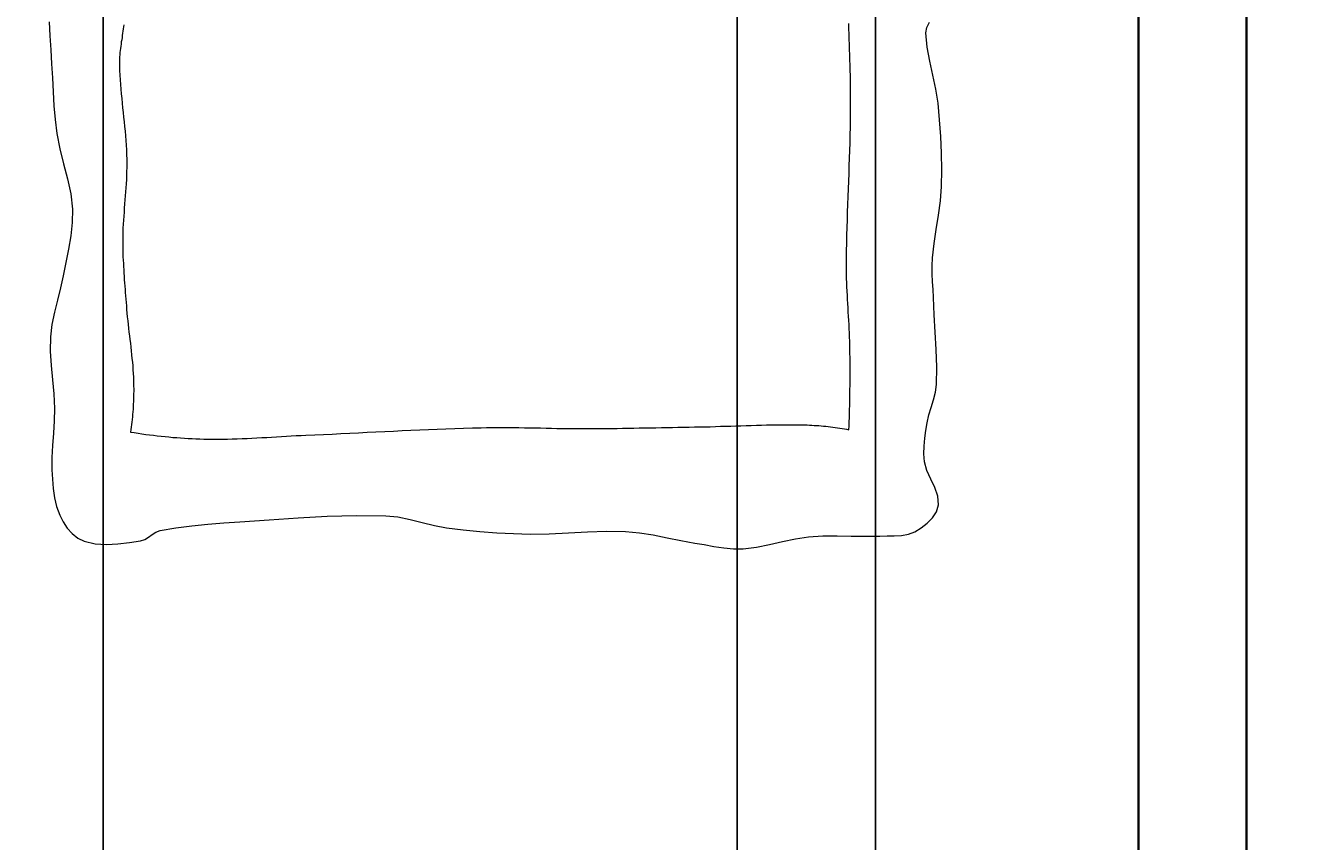
# Model space of a CAD drawing. Units: inches. Extents: x 1770 to 2988, y 1161 to 3221.
# Tile 24 of 44: x 2524 to 2631, y 2231 to 2300. Entities that reach past the tile are written whole.
import ezdxf

# ---------------------------------------------------------------- set-up
doc = ezdxf.new("R2010")
doc.units = ezdxf.units.IN
for name, color, linetype, lineweight in [('A-ANNO-DIMS', 2, 'Continuous', 18), ('A-FURN', 8, 'Continuous', 13), ('A-WALL', 7, 'Continuous', 35)]:
    doc.layers.add(name, color=color, linetype=linetype, lineweight=lineweight)
doc.styles.get("Standard").update_dxf_attribs({"font": 'arial.ttf'})
doc.dimstyles.get("Standard").update_dxf_attribs({"dimtxt": 0.18, "dimasz": 0.18, "dimexe": 0.18, "dimexo": 0.0625, "dimgap": 0.09, "dimtad": 0, "dimtih": 1, "dimtoh": 1, "dimdec": 4, "dimzin": 0, "dimdsep": 46, "dimtxsty": 'Standard', "dimcen": 0.09, "dimadec": 0, "dimazin": 0, "dimtfac": 1, "dimtdec": 4, "dimtofl": 0, "dimtmove": 0, "dimatfit": 3, "dimfxl": 1, "dimtolj": 1, "dimtzin": 0, "dimarcsym": 0})

# ---------------------------------------------------------------- blocks, each defined once
blk = doc.blocks.new('BED-DOUBLE-PLAN')
for p, q in [((0.2, 43.98), (0.26, 42.81)), ((6.33, 43.03), (6.3, 42.85)), ((6.35, 43.21), (6.33, 43.03)), ((6.37, 43.39), (6.35, 43.21)), ((6.4, 43.56), (6.37, 43.39)), ((6.42, 43.74), (6.4, 43.56)), ((66.93, 43.4), (66.91, 43.83)), ((66.94, 42.96), (66.93, 43.4)), ((73.36, 43.07), (73.44, 43.52)), ((73.46, 41.88), (73.36, 43.07)), ((73.44, 43.52), (73.64, 43.95)), ((0.26, 42.81), (0.33, 41.64)), ((6.18, 41.95), (6.15, 41.77)), ((6.2, 42.13), (6.18, 41.95)), ((6.22, 42.31), (6.2, 42.13)), ((6.25, 42.49), (6.22, 42.31)), ((6.28, 42.67), (6.25, 42.49)), ((6.3, 42.85), (6.28, 42.67)), ((66.96, 42.53), (66.94, 42.96)), ((66.97, 42.1), (66.96, 42.53)), ((66.99, 41.67), (66.97, 42.1)), ((0.33, 41.64), (0.4, 40.47)), ((6.08, 41.05), (6.07, 40.87)), ((6.07, 40.87), (6.07, 40.69)), ((6.1, 41.23), (6.08, 41.05)), ((6.11, 41.41), (6.1, 41.23)), ((6.13, 41.59), (6.11, 41.41)), ((6.15, 41.77), (6.13, 41.59)), ((67, 41.23), (66.99, 41.67)), ((67.01, 40.8), (67, 41.23)), ((73.67, 40.71), (73.46, 41.88)), ((0.4, 40.47), (0.47, 39.3)), ((6.07, 40.69), (6.07, 40.51)), ((6.07, 40.51), (6.07, 40.33)), ((6.07, 40.33), (6.08, 39.93)), ((6.08, 39.93), (6.1, 39.54)), ((67.03, 40.37), (67.01, 40.8)), ((67.04, 39.93), (67.03, 40.37)), ((67.05, 39.5), (67.04, 39.93)), ((73.93, 39.54), (73.67, 40.71)), ((0.47, 39.3), (0.53, 38.14)), ((6.1, 39.54), (6.12, 39.15)), ((6.12, 39.15), (6.15, 38.76)), ((6.15, 38.76), (6.18, 38.37)), ((67.05, 39.07), (67.05, 39.5)), ((67.06, 38.64), (67.05, 39.07)), ((74.19, 38.37), (73.93, 39.54)), ((0.53, 38.14), (0.6, 36.98)), ((6.18, 38.37), (6.21, 37.98)), ((6.21, 37.98), (6.25, 37.59)), ((67.07, 38.2), (67.06, 38.64)), ((67.07, 37.77), (67.07, 38.2)), ((67.07, 37.34), (67.07, 37.77)), ((74.37, 37.19), (74.19, 38.37)), ((0.6, 36.98), (0.69, 35.82)), ((6.25, 37.59), (6.29, 37.2)), ((6.29, 37.2), (6.33, 36.81)), ((6.33, 36.81), (6.37, 36.42)), ((67.07, 36.9), (67.07, 37.34)), ((67.07, 36.47), (67.07, 36.9)), ((74.49, 35.81), (74.37, 37.19)), ((0.69, 35.82), (0.83, 34.66)), ((6.37, 36.42), (6.41, 36.02)), ((6.41, 36.02), (6.45, 35.63)), ((6.45, 35.63), (6.49, 35.24)), ((67.06, 35.18), (67.07, 35.83)), ((67.07, 35.83), (67.07, 36.47)), ((74.59, 34.41), (74.49, 35.81)), ((0.83, 34.66), (1.08, 33.39)), ((6.49, 35.24), (6.53, 34.85)), ((6.53, 34.85), (6.56, 34.46)), ((6.56, 34.46), (6.59, 34.07)), ((67.03, 33.89), (67.04, 34.54)), ((67.04, 34.54), (67.06, 35.18)), ((74.66, 33.02), (74.59, 34.41)), ((1.08, 33.39), (1.4, 32.14)), ((6.59, 34.07), (6.62, 33.68)), ((6.62, 33.68), (6.64, 33.29)), ((67.01, 33.25), (67.03, 33.89)), ((6.64, 33.29), (6.66, 32.9)), ((6.66, 32.9), (6.67, 32.5)), ((6.67, 32.5), (6.67, 32.16)), ((66.96, 31.96), (66.99, 32.61)), ((66.99, 32.61), (67.01, 33.25)), ((74.68, 31.62), (74.66, 33.02)), ((1.4, 32.14), (1.73, 30.88)), ((6.66, 31.49), (6.65, 31.15)), ((6.67, 31.83), (6.66, 31.49)), ((6.67, 32.16), (6.67, 31.83)), ((66.92, 30.67), (66.94, 31.32)), ((66.94, 31.32), (66.96, 31.96)), ((74.66, 30.23), (74.68, 31.62)), ((1.73, 30.88), (2, 29.62)), ((6.6, 30.13), (6.57, 29.79)), ((6.62, 30.47), (6.6, 30.13)), ((6.64, 30.81), (6.62, 30.47)), ((6.65, 31.15), (6.64, 30.81)), ((66.89, 30.03), (66.92, 30.67)), ((74.57, 29.03), (74.66, 30.23)), ((2, 29.62), (2.14, 28.34)), ((6.52, 29.12), (6.5, 28.78)), ((6.55, 29.46), (6.52, 29.12)), ((6.57, 29.79), (6.55, 29.46)), ((66.84, 28.74), (66.87, 29.39)), ((66.87, 29.39), (66.89, 30.03)), ((74.4, 27.84), (74.57, 29.03)), ((2.14, 28.34), (2.12, 27.22)), ((6.45, 28.1), (6.42, 27.76)), ((6.47, 28.44), (6.45, 28.1)), ((6.5, 28.78), (6.47, 28.44)), ((66.8, 27.45), (66.82, 28.1)), ((66.82, 28.1), (66.84, 28.74)), ((2.12, 27.22), (2, 26.11)), ((6.38, 27.09), (6.36, 26.75)), ((6.4, 27.42), (6.38, 27.09)), ((6.42, 27.76), (6.4, 27.42)), ((66.78, 26.81), (66.8, 27.45)), ((74.21, 26.65), (74.4, 27.84)), ((2, 26.11), (1.8, 25)), ((6.35, 26.41), (6.34, 26.07)), ((6.34, 26.07), (6.34, 25.73)), ((6.36, 26.75), (6.35, 26.41)), ((66.75, 25.52), (66.76, 26.17)), ((66.76, 26.17), (66.78, 26.81)), ((74.03, 25.47), (74.21, 26.65)), ((1.8, 25), (1.58, 23.9)), ((6.34, 25.73), (6.34, 25.46)), ((6.34, 25.46), (6.34, 25.19)), ((6.34, 25.19), (6.35, 24.91)), ((6.35, 24.91), (6.36, 24.64)), ((66.73, 24.23), (66.74, 24.88)), ((66.74, 24.88), (66.75, 25.52)), ((73.9, 24.27), (74.03, 25.47)), ((1.58, 23.9), (1.37, 22.79)), ((6.36, 24.64), (6.36, 24.37)), ((6.36, 24.37), (6.38, 24.1)), ((6.38, 24.1), (6.39, 23.82)), ((6.39, 23.82), (6.4, 23.55)), ((66.72, 23.59), (66.73, 24.23)), ((73.87, 23.61), (73.9, 24.27)), ((1.37, 22.79), (1.15, 21.77)), ((6.4, 23.55), (6.42, 23.28)), ((6.42, 23.28), (6.43, 23.01)), ((6.43, 23.01), (6.45, 22.74)), ((6.45, 22.74), (6.47, 22.46)), ((66.73, 23.24), (66.72, 23.59)), ((66.73, 22.89), (66.73, 23.24)), ((66.74, 22.55), (66.73, 22.89)), ((73.88, 22.95), (73.87, 23.61)), ((73.91, 22.29), (73.88, 22.95)), ((1.15, 21.77), (0.89, 20.76)), ((6.47, 22.46), (6.49, 22.19)), ((6.49, 22.19), (6.51, 21.92)), ((6.51, 21.92), (6.53, 21.65)), ((6.53, 21.65), (6.55, 21.38)), ((66.75, 22.2), (66.74, 22.55)), ((66.76, 21.85), (66.75, 22.2)), ((66.78, 21.5), (66.76, 21.85)), ((73.95, 21.63), (73.91, 22.29)), ((73.98, 20.97), (73.95, 21.63)), ((0.89, 20.76), (0.64, 19.74)), ((6.55, 21.38), (6.57, 21.11)), ((6.57, 21.11), (6.59, 20.83)), ((6.59, 20.83), (6.62, 20.56)), ((6.62, 20.56), (6.64, 20.29)), ((66.8, 21.15), (66.78, 21.5)), ((66.82, 20.8), (66.8, 21.15)), ((66.84, 20.46), (66.82, 20.8)), ((66.86, 20.11), (66.84, 20.46)), ((74.05, 19.52), (73.98, 20.97)), ((0.64, 19.74), (0.42, 18.72)), ((6.64, 20.29), (6.66, 19.98)), ((6.66, 19.98), (6.69, 19.66)), ((6.69, 19.66), (6.72, 19.35)), ((66.88, 19.76), (66.86, 20.11)), ((66.9, 19.41), (66.88, 19.76)), ((66.92, 19.06), (66.9, 19.41)), ((74.14, 18.07), (74.05, 19.52)), ((0.42, 18.72), (0.3, 17.69)), ((6.72, 19.35), (6.76, 19.03)), ((6.76, 19.03), (6.79, 18.72)), ((6.79, 18.72), (6.83, 18.4)), ((6.83, 18.4), (6.86, 18.09)), ((66.94, 18.72), (66.92, 19.06)), ((66.96, 18.37), (66.94, 18.72)), ((66.97, 18.02), (66.96, 18.37)), ((0.3, 17.69), (0.28, 16.5)), ((6.86, 18.09), (6.9, 17.77)), ((6.9, 17.77), (6.94, 17.46)), ((6.94, 17.46), (6.98, 17.15)), ((66.99, 17.67), (66.97, 18.02)), ((67, 17.32), (66.99, 17.67)), ((67.01, 16.97), (67, 17.32)), ((74.22, 16.62), (74.14, 18.07)), ((0.28, 16.5), (0.36, 15.3)), ((6.98, 17.15), (7.01, 16.83)), ((7.01, 16.83), (7.05, 16.52)), ((7.05, 16.52), (7.08, 16.2)), ((7.08, 16.2), (7.11, 15.89)), ((67.02, 16.63), (67.01, 16.97)), ((67.02, 16.29), (67.02, 16.63)), ((67.03, 15.96), (67.02, 16.29)), ((74.26, 15.17), (74.22, 16.62)), ((0.36, 15.3), (0.48, 14.11)), ((7.11, 15.89), (7.14, 15.57)), ((7.14, 15.57), (7.17, 15.26)), ((7.17, 15.26), (7.19, 14.94)), ((67.03, 15.62), (67.03, 15.96)), ((67.03, 15.29), (67.03, 15.62)), ((67.03, 14.95), (67.03, 15.29)), ((74.24, 13.72), (74.26, 15.17)), ((0.48, 14.11), (0.59, 12.92)), ((7.19, 14.94), (7.21, 14.63)), ((7.21, 14.63), (7.23, 14.31)), ((7.23, 14.31), (7.24, 13.99)), ((7.24, 13.99), (7.25, 13.78)), ((67.03, 14.62), (67.03, 14.95)), ((67.03, 14.29), (67.03, 14.62)), ((67.03, 13.95), (67.03, 14.29)), ((0.59, 12.92), (0.65, 11.72)), ((7.25, 13.78), (7.25, 13.57)), ((7.25, 13.57), (7.26, 13.35)), ((7.26, 13.14), (7.25, 12.93)), ((7.25, 12.93), (7.25, 12.71)), ((7.26, 13.35), (7.26, 13.14)), ((67.01, 12.61), (67.02, 12.95)), ((67.02, 13.28), (67.03, 13.62)), ((67.02, 12.95), (67.02, 13.28)), ((67.03, 13.62), (67.03, 13.95)), ((73.98, 12.43), (74.15, 13.07)), ((74.15, 13.07), (74.24, 13.72)), ((7.21, 11.86), (7.2, 11.65)), ((7.22, 12.07), (7.21, 11.86)), ((7.23, 12.29), (7.22, 12.07)), ((7.24, 12.5), (7.23, 12.29)), ((7.25, 12.71), (7.24, 12.5)), ((66.99, 11.61), (67, 11.95)), ((67, 11.95), (67.01, 12.28)), ((67.01, 12.28), (67.01, 12.61)), ((73.78, 11.8), (73.98, 12.43)), ((0.65, 11.72), (0.62, 10.69)), ((7.12, 10.8), (7.09, 10.58)), ((7.14, 11.01), (7.12, 10.8)), ((7.16, 11.22), (7.14, 11.01)), ((7.18, 11.43), (7.16, 11.22)), ((7.2, 11.65), (7.18, 11.43)), ((66.96, 10.61), (66.97, 10.94)), ((66.97, 10.94), (66.98, 11.28)), ((66.98, 11.28), (66.99, 11.61)), ((73.45, 10.52), (73.59, 11.17)), ((73.59, 11.17), (73.78, 11.8)), ((0.62, 10.69), (0.55, 9.66)), ((7.01, 9.95), (6.98, 9.74)), ((6.98, 9.74), (7.3, 9.69)), ((7.04, 10.16), (7.01, 9.95)), ((7.07, 10.37), (7.04, 10.16)), ((7.09, 10.58), (7.07, 10.37)), ((7.3, 9.69), (7.62, 9.64)), ((25.28, 9.64), (26.01, 9.68)), ((26.01, 9.68), (26.74, 9.72)), ((26.74, 9.72), (27.47, 9.75)), ((27.47, 9.75), (28.2, 9.79)), ((28.2, 9.79), (28.93, 9.82)), ((28.93, 9.82), (29.66, 9.86)), ((29.66, 9.86), (30.39, 9.89)), ((30.39, 9.89), (31.12, 9.92)), ((31.12, 9.92), (31.85, 9.95)), ((31.85, 9.95), (32.58, 9.98)), ((32.58, 9.98), (33.31, 10.01)), ((33.31, 10.01), (34.04, 10.04)), ((34.04, 10.04), (34.78, 10.06)), ((34.78, 10.06), (35.51, 10.08)), ((35.51, 10.08), (36.24, 10.1)), ((36.24, 10.1), (36.69, 10.11)), ((36.69, 10.11), (37.14, 10.12)), ((37.14, 10.12), (37.59, 10.12)), ((37.59, 10.12), (38.04, 10.12)), ((38.04, 10.12), (38.5, 10.12)), ((38.5, 10.12), (38.95, 10.11)), ((38.95, 10.11), (39.4, 10.11)), ((39.4, 10.11), (39.85, 10.1)), ((39.85, 10.1), (40.3, 10.1)), ((40.3, 10.1), (40.75, 10.09)), ((40.75, 10.09), (41.21, 10.08)), ((41.21, 10.08), (41.66, 10.07)), ((41.66, 10.07), (42.11, 10.06)), ((42.11, 10.06), (42.56, 10.05)), ((42.56, 10.05), (43.01, 10.05)), ((43.01, 10.05), (43.47, 10.04)), ((43.47, 10.04), (43.92, 10.04)), ((43.92, 10.04), (44.37, 10.03)), ((44.37, 10.03), (44.82, 10.03)), ((44.82, 10.03), (45.27, 10.03)), ((45.27, 10.03), (45.74, 10.03)), ((45.74, 10.03), (46.2, 10.04)), ((46.2, 10.04), (46.66, 10.04)), ((46.66, 10.04), (47.12, 10.05)), ((47.12, 10.05), (47.58, 10.05)), ((47.58, 10.05), (48.04, 10.06)), ((48.04, 10.06), (48.51, 10.06)), ((48.51, 10.06), (48.97, 10.07)), ((48.97, 10.07), (49.43, 10.08)), ((49.43, 10.08), (49.89, 10.09)), ((49.89, 10.09), (50.35, 10.1)), ((50.35, 10.1), (50.82, 10.1)), ((50.82, 10.1), (51.28, 10.11)), ((51.28, 10.11), (51.74, 10.12)), ((51.74, 10.12), (52.2, 10.13)), ((52.2, 10.13), (52.66, 10.14)), ((52.66, 10.14), (53.12, 10.15)), ((53.12, 10.15), (53.59, 10.16)), ((53.59, 10.16), (54.05, 10.17)), ((54.05, 10.17), (54.51, 10.17)), ((54.51, 10.17), (54.94, 10.18)), ((54.94, 10.18), (55.36, 10.19)), ((55.36, 10.19), (55.79, 10.2)), ((55.79, 10.2), (56.22, 10.22)), ((56.22, 10.22), (56.64, 10.23)), ((56.64, 10.23), (57.07, 10.24)), ((57.07, 10.24), (57.5, 10.26)), ((57.5, 10.26), (57.92, 10.27)), ((57.92, 10.27), (58.35, 10.28)), ((58.35, 10.28), (58.78, 10.3)), ((58.78, 10.3), (59.21, 10.31)), ((59.21, 10.31), (59.63, 10.32)), ((59.63, 10.32), (60.06, 10.33)), ((60.06, 10.33), (60.49, 10.34)), ((60.49, 10.34), (60.91, 10.34)), ((60.91, 10.34), (61.34, 10.35)), ((61.34, 10.35), (61.77, 10.35)), ((61.77, 10.35), (62.19, 10.35)), ((62.19, 10.35), (62.62, 10.35)), ((62.62, 10.35), (63.05, 10.34)), ((63.05, 10.34), (63.24, 10.34)), ((63.24, 10.34), (63.44, 10.33)), ((63.44, 10.33), (63.63, 10.32)), ((63.63, 10.32), (63.83, 10.31)), ((63.83, 10.31), (64.02, 10.3)), ((64.02, 10.3), (64.22, 10.29)), ((64.22, 10.29), (64.41, 10.28)), ((64.41, 10.28), (64.61, 10.26)), ((64.61, 10.26), (64.8, 10.24)), ((64.8, 10.24), (65, 10.22)), ((65, 10.22), (65.19, 10.2)), ((65.19, 10.2), (65.39, 10.18)), ((65.39, 10.18), (65.58, 10.15)), ((65.58, 10.15), (65.78, 10.13)), ((65.78, 10.13), (65.97, 10.1)), ((65.97, 10.1), (66.16, 10.07)), ((66.16, 10.07), (66.36, 10.04)), ((66.36, 10.04), (66.55, 10.01)), ((66.55, 10.01), (66.74, 9.98)), ((66.74, 9.98), (66.93, 9.94)), ((66.93, 9.94), (66.95, 10.27)), ((66.95, 10.27), (66.96, 10.61)), ((73.26, 9.22), (73.35, 9.87)), ((73.35, 9.87), (73.45, 10.52)), ((0.47, 8.63), (0.41, 7.61)), ((0.55, 9.66), (0.47, 8.63)), ((7.62, 9.64), (7.94, 9.59)), ((7.94, 9.59), (8.26, 9.55)), ((8.26, 9.55), (8.58, 9.5)), ((8.58, 9.5), (8.9, 9.47)), ((8.9, 9.47), (9.22, 9.43)), ((9.22, 9.43), (9.55, 9.39)), ((9.55, 9.39), (9.87, 9.36)), ((9.87, 9.36), (10.19, 9.33)), ((10.19, 9.33), (10.51, 9.3)), ((10.51, 9.3), (10.84, 9.28)), ((10.84, 9.28), (11.16, 9.25)), ((11.16, 9.25), (11.48, 9.23)), ((11.48, 9.23), (11.81, 9.21)), ((11.81, 9.21), (12.13, 9.2)), ((12.13, 9.2), (12.45, 9.18)), ((12.45, 9.18), (12.78, 9.17)), ((12.78, 9.17), (13.1, 9.16)), ((13.1, 9.16), (13.43, 9.15)), ((13.43, 9.15), (13.84, 9.15)), ((13.84, 9.15), (14.25, 9.15)), ((14.25, 9.15), (14.66, 9.15)), ((14.66, 9.15), (15.07, 9.16)), ((15.07, 9.16), (15.48, 9.17)), ((15.48, 9.17), (15.89, 9.18)), ((15.89, 9.18), (16.3, 9.2)), ((16.3, 9.2), (16.71, 9.21)), ((16.71, 9.21), (17.12, 9.23)), ((17.12, 9.23), (17.53, 9.25)), ((17.53, 9.25), (17.94, 9.28)), ((17.94, 9.28), (18.35, 9.3)), ((18.35, 9.3), (18.76, 9.32)), ((18.76, 9.32), (19.17, 9.35)), ((19.17, 9.35), (19.58, 9.37)), ((19.58, 9.37), (19.99, 9.4)), ((19.99, 9.4), (20.4, 9.42)), ((20.4, 9.42), (20.81, 9.44)), ((20.81, 9.44), (21.22, 9.46)), ((21.22, 9.46), (21.63, 9.48)), ((21.63, 9.48), (22.36, 9.51)), ((22.36, 9.51), (23.09, 9.54)), ((23.09, 9.54), (23.82, 9.57)), ((23.82, 9.57), (24.55, 9.61)), ((24.55, 9.61), (25.28, 9.64)), ((73.2, 8.56), (73.26, 9.22)), ((0.41, 7.61), (0.42, 6.58)), ((73.19, 7.91), (73.2, 8.56)), ((73.24, 7.26), (73.19, 7.91)), ((0.42, 6.58), (0.47, 5.81)), ((73.44, 6.52), (73.24, 7.26)), ((73.77, 5.81), (73.44, 6.52)), ((0.47, 5.81), (0.53, 5.03)), ((74.11, 5.1), (73.77, 5.81)), ((0.53, 5.03), (0.65, 4.26)), ((74.36, 4.39), (74.11, 5.1)), ((74.4, 3.66), (74.36, 4.39)), ((0.65, 4.26), (0.82, 3.52)), ((0.82, 3.52), (1.09, 2.8)), ((74.23, 3.09), (74.4, 3.66)), ((1.09, 2.8), (1.37, 2.25)), ((1.37, 2.25), (1.71, 1.73)), ((13.44, 2.06), (14.78, 2.16)), ((14.78, 2.16), (16.12, 2.26)), ((16.12, 2.26), (18.55, 2.42)), ((18.55, 2.42), (20.98, 2.58)), ((20.98, 2.58), (23.41, 2.71)), ((23.41, 2.71), (25.85, 2.78)), ((25.85, 2.78), (28.28, 2.76)), ((28.28, 2.76), (29.3, 2.66)), ((29.3, 2.66), (30.32, 2.45)), ((30.32, 2.45), (31.33, 2.18)), ((31.33, 2.18), (32.34, 1.93)), ((73.46, 2.13), (73.9, 2.58)), ((73.9, 2.58), (74.23, 3.09)), ((1.71, 1.73), (2.12, 1.26)), ((2.12, 1.26), (2.59, 0.88)), ((8.49, 0.96), (8.8, 1.19)), ((8.8, 1.19), (9.11, 1.39)), ((9.11, 1.39), (9.46, 1.52)), ((9.46, 1.52), (10.78, 1.74)), ((10.78, 1.74), (12.11, 1.92)), ((12.11, 1.92), (13.44, 2.06)), ((32.34, 1.93), (33.36, 1.75)), ((33.36, 1.75), (34.75, 1.58)), ((34.75, 1.58), (36.14, 1.45)), ((36.14, 1.45), (37.54, 1.34)), ((37.54, 1.34), (38.94, 1.26)), ((38.94, 1.26), (40.34, 1.22)), ((40.34, 1.22), (41.93, 1.24)), ((41.93, 1.24), (43.52, 1.32)), ((43.52, 1.32), (45.12, 1.42)), ((45.12, 1.42), (46.71, 1.48)), ((46.71, 1.48), (48.3, 1.45)), ((48.3, 1.45), (49.46, 1.34)), ((49.46, 1.34), (50.61, 1.15)), ((50.61, 1.15), (51.76, 0.91)), ((70.11, 1.07), (70.71, 1.08)), ((70.71, 1.08), (71.31, 1.11)), ((71.31, 1.11), (71.89, 1.21)), ((71.89, 1.21), (72.43, 1.42)), ((72.43, 1.42), (72.96, 1.74)), ((72.96, 1.74), (73.46, 2.13)), ((2.59, 0.88), (3.12, 0.62)), ((3.12, 0.62), (4.04, 0.42)), ((4.04, 0.42), (4.98, 0.36)), ((4.98, 0.36), (5.93, 0.41)), ((5.93, 0.41), (6.89, 0.52)), ((6.89, 0.52), (7.83, 0.65)), ((7.83, 0.65), (8.17, 0.76)), ((8.17, 0.76), (8.49, 0.96)), ((51.76, 0.91), (52.9, 0.68)), ((52.9, 0.68), (54.06, 0.48)), ((54.06, 0.48), (54.86, 0.35)), ((54.86, 0.35), (55.67, 0.2)), ((55.67, 0.2), (56.48, 0.08)), ((56.48, 0.08), (57.3, 0)), ((57.3, 0), (58.11, 0)), ((58.11, 0), (59.21, 0.13)), ((59.21, 0.13), (60.3, 0.35)), ((60.3, 0.35), (61.39, 0.6)), ((61.39, 0.6), (62.47, 0.84)), ((62.47, 0.84), (63.57, 1)), ((63.57, 1), (64.76, 1.07)), ((64.76, 1.07), (65.95, 1.07)), ((65.95, 1.07), (67.13, 1.05)), ((67.13, 1.05), (68.32, 1.04)), ((68.32, 1.04), (69.51, 1.06)), ((69.51, 1.06), (70.11, 1.07))]:
    blk.add_line(p, q)
blk = doc.blocks.new('*D61')
at = {"layer": 'A-ANNO-DIMS', "color": 0, "lineweight": -2, "transparency": 16777216}
for p, q in [((2625.76, 2376.7), (2866.87, 2376.7)), ((2866.69, 2376.52), (2866.69, 1993.63)), ((2866.69, 1610.38), (2866.69, 1993.27)), ((2625.76, 1610.2), (2866.87, 1610.2))]:
    blk.add_line(p, q, dxfattribs=at)
at = {"layer": 'A-ANNO-DIMS', "color": 0, "transparency": 16777216}
for points in [[(2866.66, 2376.52), (2866.72, 2376.52), (2866.69, 2376.7)], [(2866.66, 1610.38), (2866.72, 1610.38), (2866.69, 1610.2)]]:
    blk.add_solid(points, dxfattribs=at)
at = {"layer": 'Defpoints', "color": 0, "transparency": 16777216}
for p in [(2625.7, 2376.7), (2866.69, 2376.7), (2625.7, 1610.2)]:
    blk.add_point(p, dxfattribs=at)
at = {"layer": 'A-ANNO-DIMS', "color": 0, "transparency": 16777216, "insert": (2866.69, 1993.45), "char_height": 0.18, "attachment_point": 5}
blk.add_mtext('\\A1;766.5', dxfattribs=at)
blk = doc.blocks.new('*D82')
at = {"layer": 'A-ANNO-DIMS', "color": 0, "lineweight": -2, "transparency": 16777216}
for p, q in [((2443.39, 1610.26), (2443.39, 2570.7)), ((2443.57, 2570.52), (2486.45, 2570.52)), ((2530.12, 2570.52), (2487.24, 2570.52)), ((2530.3, 1610.26), (2530.3, 2570.7))]:
    blk.add_line(p, q, dxfattribs=at)
at = {"layer": 'A-ANNO-DIMS', "color": 0, "transparency": 16777216}
for points in [[(2443.57, 2570.55), (2443.57, 2570.49), (2443.39, 2570.52)], [(2530.12, 2570.55), (2530.12, 2570.49), (2530.3, 2570.52)]]:
    blk.add_solid(points, dxfattribs=at)
at = {"layer": 'Defpoints', "color": 0, "transparency": 16777216}
for p in [(2530.3, 2570.52), (2443.39, 1610.2), (2530.3, 1610.2)]:
    blk.add_point(p, dxfattribs=at)
at = {"layer": 'A-ANNO-DIMS', "color": 0, "transparency": 16777216, "insert": (2486.85, 2570.52), "char_height": 0.18, "attachment_point": 5}
blk.add_mtext('\\A1;86.92', dxfattribs=at)
blk = doc.blocks.new('*D84')
at = {"layer": 'A-ANNO-DIMS', "color": 0, "lineweight": -2, "transparency": 16777216}
for p, q in [((2513.2, 1835.26), (2513.2, 2570.7)), ((2513.38, 2570.52), (2564.56, 2570.52)), ((2616.52, 2570.52), (2565.33, 2570.52)), ((2616.7, 1835.26), (2616.7, 2570.7))]:
    blk.add_line(p, q, dxfattribs=at)
at = {"layer": 'A-ANNO-DIMS', "color": 0, "transparency": 16777216}
for points in [[(2513.38, 2570.55), (2513.38, 2570.49), (2513.2, 2570.52)], [(2616.52, 2570.55), (2616.52, 2570.49), (2616.7, 2570.52)]]:
    blk.add_solid(points, dxfattribs=at)
at = {"layer": 'Defpoints', "color": 0, "transparency": 16777216}
for p in [(2616.7, 2570.52), (2513.2, 1835.2), (2616.7, 1835.2)]:
    blk.add_point(p, dxfattribs=at)
at = {"layer": 'A-ANNO-DIMS', "color": 0, "transparency": 16777216, "insert": (2564.95, 2570.52), "char_height": 0.18, "attachment_point": 5}
blk.add_mtext('\\A1;103.5', dxfattribs=at)
blk = doc.blocks.new('*D86')
at = {"layer": 'A-ANNO-DIMS', "color": 0, "lineweight": -2, "transparency": 16777216}
for p, q in [((2583.2, 1775.21), (2583.2, 2570.7)), ((2583.38, 2570.52), (2599.62, 2570.52)), ((2616.52, 2570.52), (2600.27, 2570.52)), ((2616.7, 1775.26), (2616.7, 2570.7))]:
    blk.add_line(p, q, dxfattribs=at)
at = {"layer": 'A-ANNO-DIMS', "color": 0, "transparency": 16777216}
for points in [[(2583.38, 2570.55), (2583.38, 2570.49), (2583.2, 2570.52)], [(2616.52, 2570.55), (2616.52, 2570.49), (2616.7, 2570.52)]]:
    blk.add_solid(points, dxfattribs=at)
at = {"layer": 'Defpoints', "color": 0, "transparency": 16777216}
for p in [(2616.7, 2570.52), (2583.2, 1775.15), (2616.7, 1775.2)]:
    blk.add_point(p, dxfattribs=at)
at = {"layer": 'A-ANNO-DIMS', "color": 0, "transparency": 16777216, "insert": (2599.95, 2570.52), "char_height": 0.18, "attachment_point": 5}
blk.add_mtext('\\A1;33.5', dxfattribs=at)
blk = doc.blocks.new('*D87')
at = {"layer": 'A-ANNO-DIMS', "color": 0, "lineweight": -2, "transparency": 16777216}
for p, q in [((2594.75, 1861.4), (2594.75, 2570.7)), ((2594.93, 2570.52), (2605.33, 2570.52)), ((2616.52, 2570.52), (2606.12, 2570.52)), ((2616.7, 1839.76), (2616.7, 2570.7))]:
    blk.add_line(p, q, dxfattribs=at)
at = {"layer": 'A-ANNO-DIMS', "color": 0, "transparency": 16777216}
for points in [[(2594.93, 2570.55), (2594.93, 2570.49), (2594.75, 2570.52)], [(2616.52, 2570.55), (2616.52, 2570.49), (2616.7, 2570.52)]]:
    blk.add_solid(points, dxfattribs=at)
at = {"layer": 'Defpoints', "color": 0, "transparency": 16777216}
for p in [(2616.7, 2570.52), (2594.75, 1861.34), (2616.7, 1839.7)]:
    blk.add_point(p, dxfattribs=at)
at = {"layer": 'A-ANNO-DIMS', "color": 0, "transparency": 16777216, "insert": (2605.72, 2570.52), "char_height": 0.18, "attachment_point": 5}
blk.add_mtext('\\A1;21.95', dxfattribs=at)

msp = doc.modelspace()

# ---------------------------------------------------------------- linework, layer by layer
at = {"layer": 'A-WALL'}
for p, q in [((2625.696, 2376.7021), (2625.696, 1610.2021)), ((2616.696, 2367.7021), (2616.696, 2175.7021))]:
    msp.add_line(p, q, dxfattribs=at)

# ---------------------------------------------------------------- block references
at = {"layer": 'A-FURN'}
msp.add_blockref('BED-DOUBLE-PLAN', (2525.5949, 2255.9126), dxfattribs=at)

# ---------------------------------------------------------------- dimensions: what is measured, and where the dimension line sits
at = {"layer": 'A-ANNO-DIMS'}
for base, p1, p2, override, picture, middle in [((2530.3038, 2570.5247), (2443.3863, 1610.2021), (2530.3038, 1610.2021), {"dimdec": 2, "dimlfac": 1, "dimrnd": 0, "dimzin": 0, "dimdsep": 46, "dimlunit": 2}, '*D82', (2486.8451, 2570.5247)), ((2616.696, 2570.5247), (2513.196, 1835.2021), (2616.696, 1835.2021), {"dimdec": 1, "dimlfac": 1, "dimrnd": 0, "dimzin": 0, "dimdsep": 46, "dimlunit": 2}, '*D84', (2564.946, 2570.5247)), ((2616.696, 2570.5247), (2583.196, 1775.149), (2616.696, 1775.2021), {"dimdec": 1, "dimlfac": 1, "dimrnd": 0, "dimzin": 0, "dimdsep": 46, "dimlunit": 2}, '*D86', (2599.946, 2570.5247)), ((2616.696, 2570.5247), (2594.7479, 1861.3395), (2616.696, 1839.7021), {"dimdec": 2, "dimlfac": 1, "dimrnd": 0, "dimzin": 0, "dimdsep": 46, "dimlunit": 2}, '*D87', (2605.7219, 2570.5247))]:
    dim = msp.add_linear_dim(base=base, p1=p1, p2=p2, dimstyle='Standard', override=override, dxfattribs=at)
    dim.commit()
    dim.dimension.update_dxf_attribs({"geometry": picture, "text_midpoint": middle})
dim = msp.add_linear_dim(base=(2866.6874, 2376.7021), p1=(2625.696, 1610.2021), p2=(2625.696, 2376.7021), angle=90, dimstyle='Standard', override={"dimdec": 1, "dimlfac": 1, "dimrnd": 0, "dimzin": 0, "dimdsep": 46, "dimlunit": 2}, dxfattribs=at)
dim.commit()
dim.dimension.update_dxf_attribs({"geometry": '*D61', "text_midpoint": (2866.6874, 1993.4521)})

doc.saveas('drawing.dxf')
